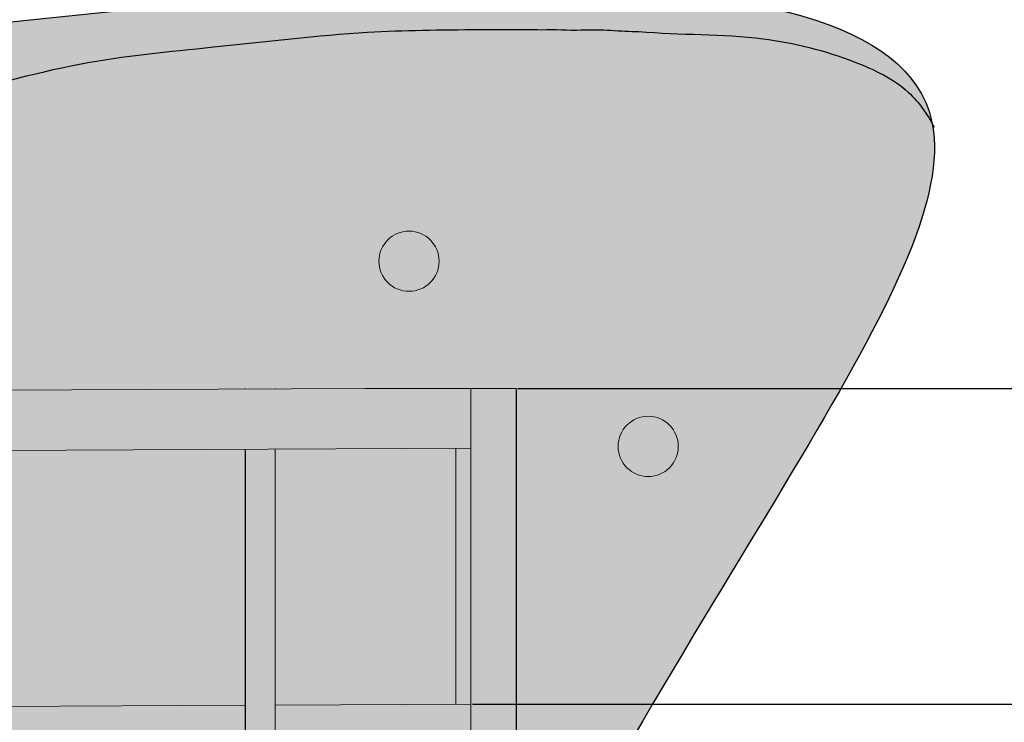
# Model space of a CAD drawing. Units: millimetres. Extents: x 11032 to 26788, y 3406 to 24505.
# Tile 73 of 78: x 21249 to 24519, y 15110 to 17443. Entities that reach past the tile are written whole.
import ezdxf

# ---------------------------------------------------------------- set-up
doc = ezdxf.new("R2010")
doc.units = ezdxf.units.MM
doc.header["$MEASUREMENT"] = 0
for name, color, linetype, lineweight in [('A-ANNO-DIMS', 2, 'Continuous', 18), ('A-GLAZ', 250, 'Continuous', 20), ('A-GLAZ-PATT', 9, 'Continuous', 13), ('A-ROOF', 7, 'Continuous', 30), ('E-LITE', 7, 'Continuous', 18), ('E-LITE-PATT', 7, 'Continuous', 13)]:
    doc.layers.add(name, color=color, linetype=linetype, lineweight=lineweight)
doc.layers.add('A-GLAZ-FRAM-PATT', color=250, linetype='Continuous', lineweight=13, true_color=0x262627)
doc.layers.add('A-ROOF-PATT', color=9, linetype='Continuous', lineweight=13, true_color=0xc7c8ca)
doc.styles.get("Standard").update_dxf_attribs({"font": 'arial.ttf'})
doc.dimstyles.get("Standard").update_dxf_attribs({"dimtxt": 150, "dimasz": 100, "dimexe": 10, "dimexo": 5, "dimgap": 5, "dimtad": 0, "dimtih": 1, "dimtoh": 1, "dimdec": 0, "dimzin": 0, "dimdsep": 46, "dimtxsty": 'Standard', "dimcen": 0.09, "dimadec": 0, "dimazin": 0, "dimtfac": 1, "dimtdec": 0, "dimtofl": 0, "dimtmove": 0, "dimatfit": 3, "dimfxl": 1, "dimtolj": 1, "dimtzin": 0, "dimarcsym": 0})

# ---------------------------------------------------------------- blocks, each defined once
blk = doc.blocks.new('RECESSED-LIGHT-200')
blk.add_circle((100, 100), 100)
blk = doc.blocks.new('*D36')
at = {"layer": 'A-ANNO-DIMS', "color": 0, "lineweight": -2, "transparency": 16777216}
for p, q in [((12301.3, 17115.9), (12301.3, 24416.9)), ((12401.3, 24406.9), (18569.2, 24406.9)), ((25297.4, 24406.9), (19129.5, 24406.9)), ((25397.4, 4466.4), (25397.4, 24416.9))]:
    blk.add_line(p, q, dxfattribs=at)
at = {"layer": 'A-ANNO-DIMS', "color": 0, "transparency": 16777216}
for points in [[(12401.3, 24423.5), (12401.3, 24390.2), (12301.3, 24406.9)], [(25297.4, 24423.5), (25297.4, 24390.2), (25397.4, 24406.9)]]:
    blk.add_solid(points, dxfattribs=at)
at = {"layer": 'Defpoints', "color": 0, "transparency": 16777216}
for p in [(25397.4, 24406.9), (12301.3, 17110.9), (25397.4, 4461.4)]:
    blk.add_point(p, dxfattribs=at)
at = {"layer": 'A-ANNO-DIMS', "color": 0, "transparency": 16777216, "insert": (18849.3, 24406.9), "char_height": 150, "attachment_point": 5}
blk.add_mtext('\\A1;13096', dxfattribs=at)
blk = doc.blocks.new('*D43')
at = {"layer": 'A-ANNO-DIMS', "color": 0, "lineweight": -2, "transparency": 16777216}
for p, q in [((22752.4, 15170.1), (26363.9, 15170.1)), ((26353.9, 15070.1), (26353.9, 14326.7)), ((26353.9, 13420.1), (26353.9, 14163.5)), ((22752.4, 13320.1), (26363.9, 13320.1))]:
    blk.add_line(p, q, dxfattribs=at)
at = {"layer": 'A-ANNO-DIMS', "color": 0, "transparency": 16777216}
for points in [[(26337.2, 15070.1), (26370.6, 15070.1), (26353.9, 15170.1)], [(26337.2, 13420.1), (26370.6, 13420.1), (26353.9, 13320.1)]]:
    blk.add_solid(points, dxfattribs=at)
at = {"layer": 'Defpoints', "color": 0, "transparency": 16777216}
for p in [(22747.4, 15170.1), (26353.9, 15170.1), (22747.4, 13320.1)]:
    blk.add_point(p, dxfattribs=at)
at = {"layer": 'A-ANNO-DIMS', "color": 0, "transparency": 16777216, "insert": (26353.9, 14245.1), "char_height": 150, "attachment_point": 5}
blk.add_mtext('\\A1;1850', dxfattribs=at)
blk = doc.blocks.new('*D44')
at = {"layer": 'A-ANNO-DIMS', "color": 0, "lineweight": -2, "transparency": 16777216}
for p, q in [((22902.4, 16218.4), (26363.9, 16218.4)), ((26353.9, 16118.4), (26353.9, 15775.9)), ((26353.9, 15270.1), (26353.9, 15612.6)), ((22752.4, 15170.1), (26363.9, 15170.1))]:
    blk.add_line(p, q, dxfattribs=at)
at = {"layer": 'A-ANNO-DIMS', "color": 0, "transparency": 16777216}
for points in [[(26337.2, 16118.4), (26370.6, 16118.4), (26353.9, 16218.4)], [(26337.2, 15270.1), (26370.6, 15270.1), (26353.9, 15170.1)]]:
    blk.add_solid(points, dxfattribs=at)
at = {"layer": 'Defpoints', "color": 0, "transparency": 16777216}
for p in [(22897.4, 16218.4), (26353.9, 16218.4), (22747.4, 15170.1)]:
    blk.add_point(p, dxfattribs=at)
at = {"layer": 'A-ANNO-DIMS', "color": 0, "transparency": 16777216, "insert": (26353.9, 15694.3), "char_height": 150, "attachment_point": 5}
blk.add_mtext('\\A1;1048.3', dxfattribs=at)
blk = doc.blocks.new('*D45')
at = {"layer": 'A-ANNO-DIMS', "color": 0, "lineweight": -2, "transparency": 16777216}
for p, q in [((13792.4, 18518.9), (26363.9, 18518.9)), ((26353.9, 18418.9), (26353.9, 17450.3)), ((26353.9, 16318.4), (26353.9, 17287)), ((22902.4, 16218.4), (26363.9, 16218.4))]:
    blk.add_line(p, q, dxfattribs=at)
at = {"layer": 'A-ANNO-DIMS', "color": 0, "transparency": 16777216}
for points in [[(26337.2, 18418.9), (26370.6, 18418.9), (26353.9, 18518.9)], [(26337.2, 16318.4), (26370.6, 16318.4), (26353.9, 16218.4)]]:
    blk.add_solid(points, dxfattribs=at)
at = {"layer": 'Defpoints', "color": 0, "transparency": 16777216}
for p in [(13787.4, 18518.9), (26353.9, 18518.9), (22897.4, 16218.4)]:
    blk.add_point(p, dxfattribs=at)
at = {"layer": 'A-ANNO-DIMS', "color": 0, "transparency": 16777216, "insert": (26353.9, 17368.7), "char_height": 150, "attachment_point": 5}
blk.add_mtext('\\A1;2300.5', dxfattribs=at)
blk = doc.blocks.new('*D51')
at = {"layer": 'A-ANNO-DIMS', "color": 0, "lineweight": -2, "transparency": 16777216}
for p, q in [((19697.4, 16000.7), (19697.4, 3494.9)), ((21997.4, 16011.6), (21997.4, 3494.9)), ((19797.4, 3504.9), (20617.4, 3504.9)), ((21897.4, 3504.9), (21077.4, 3504.9))]:
    blk.add_line(p, q, dxfattribs=at)
at = {"layer": 'A-ANNO-DIMS', "color": 0, "transparency": 16777216}
for points in [[(19797.4, 3521.6), (19797.4, 3488.2), (19697.4, 3504.9)], [(21897.4, 3521.6), (21897.4, 3488.2), (21997.4, 3504.9)]]:
    blk.add_solid(points, dxfattribs=at)
at = {"layer": 'Defpoints', "color": 0, "transparency": 16777216}
for p in [(19697.4, 16005.7), (21997.4, 16016.6), (21997.4, 3504.9)]:
    blk.add_point(p, dxfattribs=at)
at = {"layer": 'A-ANNO-DIMS', "color": 0, "transparency": 16777216, "insert": (20847.4, 3504.9), "char_height": 150, "attachment_point": 5}
blk.add_mtext('\\A1;2300', dxfattribs=at)
blk = doc.blocks.new('*D52')
at = {"layer": 'A-ANNO-DIMS', "color": 0, "lineweight": -2, "transparency": 16777216}
for p, q in [((22897.4, 16213.4), (22897.4, 3494.9)), ((21997.4, 16011.6), (21997.4, 3494.9)), ((22097.4, 3504.9), (22277, 3504.9)), ((22797.4, 3504.9), (22617.9, 3504.9))]:
    blk.add_line(p, q, dxfattribs=at)
at = {"layer": 'A-ANNO-DIMS', "color": 0, "transparency": 16777216}
for points in [[(22097.4, 3521.6), (22097.4, 3488.2), (21997.4, 3504.9)], [(22797.4, 3521.6), (22797.4, 3488.2), (22897.4, 3504.9)]]:
    blk.add_solid(points, dxfattribs=at)
at = {"layer": 'Defpoints', "color": 0, "transparency": 16777216}
for p in [(22897.4, 16218.4), (21997.4, 16016.6), (22897.4, 3504.9)]:
    blk.add_point(p, dxfattribs=at)
at = {"layer": 'A-ANNO-DIMS', "color": 0, "transparency": 16777216, "insert": (22447.4, 3504.9), "char_height": 150, "attachment_point": 5}
blk.add_mtext('\\A1;900', dxfattribs=at)

msp = doc.modelspace()

# ---------------------------------------------------------------- hatches: boundary and pattern name
at = {"layer": 'A-GLAZ-FRAM-PATT'}
h = msp.add_hatch(color=256, dxfattribs=at)
h.paths.add_polyline_path([(22747.404, 16218.44), (22395.025, 16218.44), (18518.2, 16200.148), (18519.143, 16000.151), (22747.404, 16020.1)])
edge = h.paths.add_edge_path()
edge.add_line((22897.404, 16218.44), (22747.404, 16218.44))
edge.add_line((22747.404, 16218.44), (22747.404, 16020.1))
edge.add_line((22747.404, 16020.1), (22747.404, 9631.346))
edge.add_spline(control_points=[(22747.404, 9631.346), (22803.273, 9520.228), (22853.467, 9405.87), (22897.404, 9289.211)], knot_values=[2645.78092422, 2645.78092422, 2645.78092422, 2645.78092422, 3013.05623672, 3013.05623672, 3013.05623672, 3013.05623672], degree=3, periodic=0)
edge.add_line((22897.404, 9289.211), (22897.404, 16218.44))
h.paths.add_polyline_path([(22097.404, 16017.033), (21997.404, 16016.562), (21997.404, 13316.532), (22097.404, 13317.003)])
edge = h.paths.add_edge_path()
edge.add_line((19797.404, 16006.182), (19697.404, 16005.71))
edge.add_line((19697.404, 16005.71), (19697.404, 15155.703))
edge.add_line((19697.404, 15155.703), (19697.404, 12747.012))
edge.add_spline(control_points=[(19697.404, 12747.012), (19708.389, 12750.081), (19719.253, 12753.406), (19732.457, 12757.789), (19734.918, 12758.62), (19737.372, 12759.464)], knot_values=[1372.60477099, 1372.60477099, 1372.60477099, 1372.60477099, 1399.44343377, 1399.44343377, 1405.61279972, 1405.61279972, 1405.61279972, 1405.61279972], degree=3, periodic=0)
edge.add_spline(control_points=[(19737.372, 12759.464), (19750.245, 12763.891), (19762.932, 12768.657), (19778.9, 12775.14), (19782.354, 12776.572), (19785.794, 12778.028)], knot_values=[1405.61279972, 1405.61279972, 1405.61279972, 1405.61279972, 1437.96891336, 1437.96891336, 1446.94640473, 1446.94640473, 1446.94640473, 1446.94640473], degree=3, periodic=0)
edge.add_spline(control_points=[(19785.794, 12778.028), (19789.682, 12779.673), (19793.552, 12781.348), (19797.404, 12783.051)], knot_values=[1446.94640473, 1446.94640473, 1446.94640473, 1446.94640473, 1457.09545574, 1457.09545574, 1457.09545574, 1457.09545574], degree=3, periodic=0)
edge.add_line((19797.404, 12783.051), (19797.404, 15306.174))
edge.add_line((19797.404, 15306.174), (19797.404, 16006.182))
h = msp.add_hatch(color=256, dxfattribs=at)
h.paths.add_polyline_path([(22747.404, 16020.1), (22697.404, 16019.864), (22697.404, 15169.858), (22747.404, 15170.094)])
h.paths.add_polyline_path([(22747.404, 15070.092), (22697.404, 15069.857), (22697.404, 13319.834), (22747.404, 13320.07)])
edge = h.paths.add_edge_path()
edge.add_line((22747.404, 12795.064), (21365.955, 12788.546))
edge.add_spline(control_points=[(21365.955, 12788.546), (21365.556, 12785.216), (21365.14, 12781.894), (21364.707, 12778.582)], knot_values=[4871.89074498, 4871.89074498, 4871.89074498, 4871.89074498, 4881.51384723, 4881.51384723, 4881.51384723, 4881.51384723], degree=3, periodic=0)
edge.add_spline(control_points=[(21364.707, 12778.582), (21363.953, 12772.805), (21363.147, 12767.057), (21359.867, 12745.141), (21357.035, 12729.186), (21353.796, 12713.488)], knot_values=[4881.51384723, 4881.51384723, 4881.51384723, 4881.51384723, 4898.30109774, 4898.30109774, 4945.85686537, 4945.85686537, 4945.85686537, 4945.85686537], degree=3, periodic=0)
edge.add_line((21353.796, 12713.488), (22747.404, 12720.064))
edge.add_line((22747.404, 12720.064), (22747.404, 12795.064))
edge = h.paths.add_edge_path()
edge.add_line((22747.404, 13320.07), (22697.404, 13319.834))
edge.add_line((22697.404, 13319.834), (21312.567, 13313.3))
edge.add_spline(control_points=[(21312.567, 13313.3), (21312.567, 13313.3), (21312.567, 13313.3), (21312.567, 13313.3)], knot_values=[4405.86932069, 4405.86932069, 4405.86932069, 4405.86932069, 4405.86932536, 4405.86932536, 4405.86932536, 4405.86932536], degree=3, periodic=0)
edge.add_spline(control_points=[(21312.567, 13313.3), (21316.329, 13300.292), (21319.935, 13287.252), (21326.522, 13262.273), (21329.53, 13250.337), (21332.397, 13238.393)], knot_values=[4405.86932536, 4405.86932536, 4405.86932536, 4405.86932536, 4439.73791994, 4439.73791994, 4470.65028407, 4470.65028407, 4470.65028407, 4470.65028407], degree=3, periodic=0)
edge.add_line((21332.397, 13238.393), (22747.404, 13245.069))
edge.add_line((22747.404, 13245.069), (22747.404, 13320.07))
h.paths.add_polyline_path([(22747.404, 13245.069), (22697.404, 13244.833), (22697.404, 12794.828), (22747.404, 12795.064)])
h.paths.add_polyline_path([(22747.404, 12720.064), (22697.404, 12719.828), (22697.404, 11219.811), (22747.404, 11220.047)])
edge = h.paths.add_edge_path()
edge.add_line((22747.404, 11120.046), (22697.404, 11119.81))
edge.add_line((22697.404, 11119.81), (22697.404, 9727.135))
edge.add_spline(control_points=[(22697.404, 9727.135), (22714.538, 9695.493), (22731.209, 9663.555), (22747.404, 9631.346)], knot_values=[2539.32128955, 2539.32128955, 2539.32128955, 2539.32128955, 2645.78092422, 2645.78092422, 2645.78092422, 2645.78092422], degree=3, periodic=0)
edge.add_line((22747.404, 9631.346), (22747.404, 11120.046))
h = msp.add_hatch(color=256, dxfattribs=at)
h.paths.add_polyline_path([(19697.404, 15155.703), (18523.154, 15150.163), (18523.626, 15050.164), (19697.404, 15055.702)])
h.paths.add_polyline_path([(21997.404, 15166.555), (19797.404, 15156.175), (19797.404, 15056.174), (20912.335, 15061.434, -0.11801722), (20947.253, 15061.599), (21997.404, 15066.554)])
h.paths.add_polyline_path([(22747.404, 15170.094), (22097.404, 15167.027), (22097.404, 15067.026), (22747.404, 15070.092)])
edge = h.paths.add_edge_path()
edge.add_line((21997.404, 13241.531), (21332.397, 13238.393))
edge.add_spline(control_points=[(21332.397, 13238.393), (21338.038, 13214.902), (21343.139, 13191.382), (21354.5, 13132.481), (21360.029, 13097.149), (21368.306, 13027.119), (21371.052, 12992.421), (21373.63, 12924.101), (21373.462, 12890.481), (21370.61, 12834.187), (21368.665, 12811.15), (21365.955, 12788.546)], knot_values=[4470.65028407, 4470.65028407, 4470.65028407, 4470.65028407, 4531.4505555, 4531.4505555, 4623.16319106, 4623.16319106, 4714.87582662, 4714.87582662, 4806.58846218, 4806.58846218, 4871.89074498, 4871.89074498, 4871.89074498, 4871.89074498], degree=3, periodic=0)
edge.add_line((21365.955, 12788.546), (21997.404, 12791.526))
edge.add_line((21997.404, 12791.526), (21997.404, 13241.531))
h.paths.add_polyline_path([(22097.404, 13242.003), (21997.404, 13241.531), (21997.404, 12791.526), (22097.404, 12791.998)])
h.paths.add_polyline_path([(22697.404, 13244.833), (22097.404, 13242.003), (22097.404, 12791.998), (22697.404, 12794.828)])
at = {"layer": 'A-GLAZ-PATT'}
h = msp.add_hatch(color=256, dxfattribs=at)
h.set_gradient(color1=(254, 221, 154), color2=(248, 246, 176), name='CURVED')
edge = h.paths.add_edge_path()
edge.add_spline(control_points=[(18522.918, 15200.175), (18561.599, 15201.209), (18600.224, 15202.243), (18716.594, 15205.749), (18794.099, 15208.613), (18948.086, 15217.451), (19024.568, 15223.425), (19176.135, 15240.511), (19251.219, 15251.623), (19333.848, 15267.966), (19342.25, 15269.676), (19356.967, 15272.758), (19363.289, 15274.111), (19375.94, 15276.871), (19382.267, 15278.279), (19401.252, 15282.576), (19413.915, 15285.541), (19451.935, 15294.685), (19477.322, 15301.111), (19548.254, 15319.552), (19593.948, 15331.984), (19659.079, 15349.253), (19678.203, 15354.269), (19697.404, 15359.188)], knot_values=[1.09285599, 1.09285599, 1.09285599, 1.09285599, 116.34451384, 116.34451384, 349.03354152, 349.03354152, 581.72256921, 581.72256921, 814.41159689, 814.41159689, 840.78637359, 840.78637359, 860.67891922, 860.67891922, 880.57146485, 880.57146485, 920.35655611, 920.35655611, 999.92673863, 999.92673863, 1142.09604805, 1142.09604805, 1200.90860694, 1200.90860694, 1200.90860694, 1200.90860694], degree=3, periodic=0)
edge.add_line((19697.404, 15359.188), (19697.404, 16005.71))
edge.add_line((19697.404, 16005.71), (18519.143, 16000.151))
edge.add_line((18519.143, 16000.151), (18522.918, 15200.175))
edge = h.paths.add_edge_path()
edge.add_line((19697.404, 15055.702), (18523.626, 15050.164))
edge.add_line((18523.626, 15050.164), (18531.851, 13306.733))
edge.add_spline(control_points=[(18531.851, 13306.733), (18553.325, 13284.933), (18574.901, 13263.301), (18632.771, 13206.214), (18669.261, 13171.188), (18735.852, 13109.762), (18765.813, 13083.011), (18826.398, 13031.156), (18857.021, 13006.052), (18919.15, 12957.862), (18950.655, 12934.774), (19007.615, 12895.967), (19032.834, 12879.759), (19084.165, 12849.05), (19110.278, 12834.547), (19163.6, 12807.555), (19190.811, 12795.065), (19240.068, 12775.123), (19261.85, 12767.175), (19306.233, 12752.949), (19328.834, 12746.672), (19374.859, 12736.071), (19398.283, 12731.748), (19445.866, 12725.365), (19470.026, 12723.306), (19514.597, 12721.889), (19534.921, 12722.121), (19575.756, 12724.466), (19596.267, 12726.579), (19622.683, 12730.57), (19628.6, 12731.546), (19638.601, 12733.337), (19642.688, 12734.108), (19650.826, 12735.723), (19654.881, 12736.567), (19667.001, 12739.207), (19675.023, 12741.111), (19687.813, 12744.388), (19692.62, 12745.676), (19697.404, 12747.012)], knot_values=[259.28299856, 259.28299856, 259.28299856, 259.28299856, 332.45020059, 332.45020059, 454.53383699, 454.53383699, 552.84889009, 552.84889009, 651.16394319, 651.16394319, 749.47899629, 749.47899629, 825.6298474, 825.6298474, 901.7806985, 901.7806985, 977.9315496, 977.9315496, 1036.43952646, 1036.43952646, 1094.94750331, 1094.94750331, 1153.45548017, 1153.45548017, 1211.96345702, 1211.96345702, 1260.21270617, 1260.21270617, 1308.46195531, 1308.46195531, 1322.39247458, 1322.39247458, 1332.02384448, 1332.02384448, 1341.65521438, 1341.65521438, 1360.91795418, 1360.91795418, 1372.60477099, 1372.60477099, 1372.60477099, 1372.60477099], degree=3, periodic=0)
edge.add_line((19697.404, 12747.012), (19697.404, 15055.702))
h.paths.add_polyline_path([(18790.086, 14298.34, -1), (18890.086, 14298.34, -1)], flags=16)
h.paths.add_polyline_path([(19437.524, 14550.125, -1), (19537.524, 14550.125, -1)], flags=16)
h.paths.add_polyline_path([(22697.404, 16019.864), (22097.404, 16017.033), (22097.404, 15167.027), (22697.404, 15169.858)])
h.paths.add_polyline_path([(22697.404, 15069.857), (22097.404, 15067.026), (22097.404, 13317.003), (22697.404, 13319.834)])
h.paths.add_polyline_path([(20866.429, 15795.606, -1), (21016.429, 15795.606, -1)], flags=16)
h.paths.add_polyline_path([(19822.441, 15337.78), (19797.404, 15332.147), (19797.404, 15156.175), (20721.869, 15160.537), (20700.803, 15175.665), (20679.512, 15190.548), (20657.993, 15205.143), (20636.247, 15219.41), (20614.273, 15233.307), (20592.07, 15246.794), (20569.639, 15259.829), (20546.978, 15272.372), (20524.088, 15284.38), (20500.968, 15295.814), (20477.616, 15306.631), (20454.034, 15316.792), (20430.219, 15326.254), (20406.173, 15334.976), (20381.894, 15342.919), (20357.382, 15350.039), (20332.636, 15356.297), (20307.662, 15361.667), (20282.483, 15366.173), (20257.125, 15369.849), (20231.617, 15372.729), (20205.984, 15374.847), (20180.253, 15376.236), (20154.451, 15376.931), (20128.605, 15376.964), (20102.742, 15376.37), (20076.889, 15375.183), (20051.072, 15373.436), (20025.318, 15371.163), (19999.653, 15368.398), (19974.087, 15365.173), (19948.614, 15361.516), (19923.228, 15357.456), (19897.924, 15353.024), (19872.695, 15348.248), (19847.536, 15343.157)])
h.paths.add_polyline_path([(19797.404, 15383.428), (19822.666, 15388.998), (19848.044, 15394.311), (19873.542, 15399.338), (19899.168, 15404.048), (19924.927, 15408.41), (19950.824, 15412.396), (19976.865, 15415.972), (20003.054, 15419.109), (20029.394, 15421.774), (20055.871, 15423.934), (20082.461, 15425.553), (20109.142, 15426.594), (20135.888, 15427.02), (20162.676, 15426.794), (20189.481, 15425.88), (20216.28, 15424.237), (20243.046, 15421.828), (20269.754, 15418.614), (20296.377, 15414.554), (20322.887, 15409.61), (20349.254, 15403.74), (20375.368, 15396.947), (20401.163, 15389.283), (20426.64, 15380.795), (20451.799, 15371.531), (20476.643, 15361.538), (20501.172, 15350.863), (20525.391, 15339.55), (20549.302, 15327.645), (20572.91, 15315.192), (20596.218, 15302.234), (20619.229, 15288.816), (20641.948, 15274.978), (20664.378, 15260.764), (20686.523, 15246.215), (20708.386, 15231.373), (20729.97, 15216.279), (20751.277, 15200.974), (20806.33, 15160.935), (21997.404, 15166.555), (21997.404, 16016.562), (19797.404, 16006.182)])
at = {"layer": 'A-ROOF-PATT'}
h = msp.add_hatch(color=256, dxfattribs=at)
edge = h.paths.add_edge_path()
edge.add_spline(control_points=[(18514.126, 17063.566), (18809.773, 17038.521), (19288.07, 16988.339), (19761.843, 17020.464), (19965.955, 17031.58)], knot_values=[0, 0, 0, 0, 871.48115533, 1383.18424693, 1383.18424693, 1383.18424693, 1383.18424693], degree=3, periodic=0)
edge.add_spline(control_points=[(19965.955, 17031.58), (20122.484, 17046.068), (20408.011, 17091.181), (20910.567, 17150.246), (21440.234, 17310.172), (21915.866, 17351.508), (22364.272, 17406.622), (22705.353, 17409.356), (22912.577, 17410.967), (22981.194, 17409.426)], knot_values=[0, 0, 0, 0, 414.81784697, 1085.22788952, 1556.54039253, 2003.31216232, 2520.51919616, 2899.47011217, 3092.27759325, 3092.27759325, 3092.27759325, 3092.27759325], degree=3, periodic=0)
edge.add_spline(control_points=[(22981.194, 17409.426), (23026.355, 17412.719), (23070.675, 17406.134), (23179.968, 17412.17), (23244.326, 17403.734), (23304.873, 17403.391)], knot_values=[11756.28081343, 11756.28081343, 11756.28081343, 11756.28081343, 11879.15309498, 11879.15309498, 12065.87545546, 12065.87545546, 12065.87545546, 12065.87545546], degree=3, periodic=0)
edge.add_spline(control_points=[(23304.873, 17403.391), (23443.416, 17391.278), (23687.5, 17400.339), (23988.629, 17323.661), (24193.084, 17226.949), (24257.37, 17136.735), (24279.347, 17098.191)], knot_values=[0, 0, 0, 0, 412.75172359, 727.19040018, 931.86025321, 1064.01641738, 1064.01641738, 1064.01641738, 1064.01641738], degree=3, periodic=0)
edge.add_spline(control_points=[(24279.347, 17098.191), (24276.632, 17112.026), (24103.56, 17784.539), (21679.83, 17482.933), (20092.886, 17311.864), (19886.51, 17298.161)], knot_values=[9435.32329041, 9435.32329041, 9435.32329041, 9435.32329041, 9511.54858978, 13244.41643911, 13837.11981978, 13837.11981978, 13837.11981978, 13837.11981978], degree=3, periodic=0)
edge.add_spline(control_points=[(19886.51, 17298.161), (19770.33, 17290.447), (19654.15, 17282.732), (19537.97, 17275.018), (19460.41, 17269.868), (19382.851, 17264.718), (19305.291, 17259.568)], knot_values=[8878.9087223, 8878.9087223, 8878.9087223, 8878.9087223, 9212.57342317, 9212.57342317, 9212.57342317, 9435.32303857, 9435.32303857, 9435.32303857, 9435.32303857], degree=3, periodic=0)
edge.add_spline(control_points=[(19305.291, 17259.568), (19183.371, 17255.041), (18919.19, 17257.277), (18655.158, 17260.282), (18513.182, 17263.662)], knot_values=[568.98430855, 568.98430855, 568.98430855, 568.98430855, 934.97323186, 1361.07600794, 1361.07600794, 1361.07600794, 1361.07600794], degree=3, periodic=0)
edge.add_line((18513.182, 17263.662), (18514.126, 17063.566))
h = msp.add_hatch(color=256, dxfattribs=at)
h.set_gradient(color1=(254, 234, 185), color2=(254, 204, 102), name='HEMISPHERICAL')
edge = h.paths.add_edge_path()
edge.add_line((22395.025, 16218.44), (22897.404, 16218.44))
edge.add_line((22897.404, 16218.44), (22897.404, 14361.22))
edge.add_spline(control_points=[(22897.404, 14361.22), (23633.498, 15762.375), (24369.592, 16638.387), (24279.347, 17098.191)], knot_values=[13837.11981978, 13837.11981978, 13837.11981978, 13837.11981978, 16370.50452639, 16370.50452639, 16370.50452639, 16370.50452639], degree=3, periodic=0)
edge.add_spline(control_points=[(24279.347, 17098.191), (24257.37, 17136.735), (24193.084, 17226.949), (23988.629, 17323.661), (23687.5, 17400.339), (23443.416, 17391.278), (23304.873, 17403.391)], knot_values=[0, 0, 0, 0, 132.15616417, 336.8260172, 651.2646938, 1064.01641738, 1064.01641738, 1064.01641738, 1064.01641738], degree=3, periodic=0)
edge.add_spline(control_points=[(23304.873, 17403.391), (23244.326, 17403.734), (23179.968, 17412.17), (23070.675, 17406.134), (23026.355, 17412.719), (22981.194, 17409.426)], knot_values=[11756.28081343, 11756.28081343, 11756.28081343, 11756.28081343, 11943.0031739, 11943.0031739, 12065.87545546, 12065.87545546, 12065.87545546, 12065.87545546], degree=3, periodic=0)
edge.add_spline(control_points=[(22981.194, 17409.426), (22912.577, 17410.967), (22705.353, 17409.356), (22364.272, 17406.622), (21915.866, 17351.508), (21440.234, 17310.172), (20910.567, 17150.246), (20408.011, 17091.181), (20122.484, 17046.068), (19965.955, 17031.58)], knot_values=[0, 0, 0, 0, 192.80748108, 571.75839709, 1088.96543094, 1535.73720072, 2007.04970373, 2677.45974628, 3092.27759325, 3092.27759325, 3092.27759325, 3092.27759325], degree=3, periodic=0)
edge.add_spline(control_points=[(19965.955, 17031.58), (19761.843, 17020.464), (19288.07, 16988.339), (18809.773, 17038.521), (18514.126, 17063.566)], knot_values=[0, 0, 0, 0, 511.7030916, 1383.18424693, 1383.18424693, 1383.18424693, 1383.18424693], degree=3, periodic=0)
edge.add_line((18514.126, 17063.566), (18518.2, 16200.148))
edge.add_line((18518.2, 16200.148), (22395.025, 16218.44))
h.paths.add_polyline_path([(20159.481, 16629.671, -1), (20359.481, 16629.671, -1)], flags=16)
h.paths.add_polyline_path([(22641.869, 16640.848, -1), (22441.869, 16640.848, -1)], flags=16)
h.paths.add_polyline_path([(23436.23, 16026.079, -1), (23236.23, 16026.079, -1)], flags=16)
at = {"layer": 'E-LITE-PATT'}
h = msp.add_hatch(color=256, dxfattribs=at)
edge = h.paths.add_edge_path()
edge.add_spline(control_points=[(18523.154, 15150.163), (18807.347, 15157.761), (19206.112, 15168.423), (19587.098, 15279.026), (19697.404, 15307.557)], knot_values=[0, 0, 0, 0, 846.75149574, 1188.1141131, 1188.1141131, 1188.1141131, 1188.1141131], degree=3, periodic=0)
edge.add_line((19697.404, 15307.557), (19697.404, 15359.188))
edge.add_spline(control_points=[(19697.404, 15359.188), (19678.203, 15354.269), (19659.079, 15349.253), (19593.948, 15331.984), (19548.254, 15319.552), (19477.322, 15301.111), (19451.935, 15294.685), (19413.915, 15285.541), (19401.252, 15282.576), (19382.267, 15278.279), (19375.94, 15276.871), (19363.289, 15274.111), (19356.967, 15272.758), (19342.25, 15269.676), (19333.848, 15267.966), (19251.219, 15251.623), (19176.135, 15240.511), (19024.568, 15223.425), (18948.086, 15217.451), (18794.099, 15208.613), (18716.594, 15205.749), (18600.224, 15202.243), (18561.599, 15201.209), (18522.918, 15200.175)], knot_values=[1.09285599, 1.09285599, 1.09285599, 1.09285599, 59.90541488, 59.90541488, 202.0747243, 202.0747243, 281.64490682, 281.64490682, 321.42999808, 321.42999808, 341.32254371, 341.32254371, 361.21508934, 361.21508934, 387.58986604, 387.58986604, 620.27889372, 620.27889372, 852.96792141, 852.96792141, 1085.65694909, 1085.65694909, 1200.90860694, 1200.90860694, 1200.90860694, 1200.90860694], degree=3, periodic=0)
edge.add_line((18522.918, 15200.175), (18523.154, 15150.163))
edge = h.paths.add_edge_path()
edge.add_spline(control_points=[(19797.404, 15332.147), (19868.636, 15348.527), (20045.965, 15382.128), (20379.232, 15379.049), (20603.72, 15246.463), (20721.869, 15160.537)], knot_values=[1290.96802179, 1290.96802179, 1290.96802179, 1290.96802179, 1509.98304384, 1831.38750258, 2265.00925431, 2265.00925431, 2265.00925431, 2265.00925431], degree=3, periodic=0)
edge.add_line((20721.869, 15160.537), (20806.33, 15160.935))
edge.add_spline(control_points=[(20806.33, 15160.935), (20787.979, 15174.281), (20769.629, 15187.627), (20751.278, 15200.973), (20751.278, 15200.973), (20751.277, 15200.974), (20751.277, 15200.974)], knot_values=[2265.00925431, 2265.00925431, 2265.00925431, 2265.00925431, 2330.89307837, 2330.89307837, 2330.89307837, 2330.89358007, 2330.89358007, 2330.89358007, 2330.89358007], degree=3, periodic=0)
edge.add_spline(control_points=[(20751.277, 15200.974), (20751.247, 15200.996), (20751.217, 15201.018), (20722.252, 15222.081), (20692.553, 15242.645), (20631.556, 15281.877), (20600.258, 15300.544), (20535.977, 15335.007), (20502.992, 15350.803), (20448.844, 15372.942), (20428.246, 15380.535), (20396.869, 15390.701), (20386.329, 15393.886), (20370.401, 15398.335), (20365.072, 15399.763), (20354.373, 15402.506), (20349.001, 15403.822), (20337.544, 15406.494), (20331.459, 15407.834), (20315.169, 15411.216), (20304.944, 15413.125), (20281.909, 15416.972), (20269.086, 15418.802), (20222.263, 15424.425), (20188.116, 15426.504), (20124.362, 15427.321), (20094.738, 15426.456), (20050.592, 15423.632), (20035.925, 15422.435), (20006.724, 15419.587), (19992.193, 15417.937), (19959.175, 15413.705), (19940.732, 15410.994), (19880.215, 15401.109), (19838.589, 15392.722), (19797.404, 15383.428)], knot_values=[1302.24166378, 1302.24166378, 1302.24166378, 1302.24166378, 1302.35087893, 1302.35087893, 1406.225269, 1406.225269, 1510.09965908, 1510.09965908, 1613.97404916, 1613.97404916, 1676.17986117, 1676.17986117, 1707.28276717, 1707.28276717, 1722.83422018, 1722.83422018, 1738.38567318, 1738.38567318, 1755.91676333, 1755.91676333, 1785.22951081, 1785.22951081, 1821.79065604, 1821.79065604, 1918.47644845, 1918.47644845, 2002.64679624, 2002.64679624, 2044.73197014, 2044.73197014, 2086.81714404, 2086.81714404, 2140.81625119, 2140.81625119, 2265.00925431, 2265.00925431, 2265.00925431, 2265.00925431], degree=3, periodic=0)
edge.add_line((19797.404, 15383.428), (19797.404, 15332.147))
h.paths.add_polyline_path([(21016.429, 15795.606, 1), (20866.429, 15795.606, 1)])
h.paths.add_polyline_path([(23236.23, 16026.079, 1), (23436.23, 16026.079, 1)])
h.paths.add_polyline_path([(22441.869, 16640.848, 1), (22641.869, 16640.848, 1)])
h.paths.add_polyline_path([(20159.481, 16629.671, 1), (20359.481, 16629.671, 1)])

# ---------------------------------------------------------------- linework, layer by layer
at = {"layer": 'A-GLAZ'}
for p, q in [((22395.025, 16218.44), (18518.2, 16200.148)), ((21997.404, 16218.44), (21997.404, 16216.564)), ((22097.404, 16218.44), (22097.404, 16217.036)), ((22897.404, 16218.44), (22395.025, 16218.44)), ((22747.404, 16218.44), (22747.404, 9631.346)), ((22897.404, 16218.44), (22897.404, 9289.211)), ((22747.404, 16020.1), (18519.143, 16000.151)), ((21997.404, 16016.562), (21997.404, 13316.532)), ((22097.404, 16017.033), (22097.404, 13317.003)), ((22697.404, 16019.864), (22697.404, 15169.858)), ((22697.404, 15319.857), (22697.404, 15169.858)), ((21997.404, 15166.555), (19797.404, 15156.175)), ((22747.404, 15170.094), (22097.404, 15167.027))]:
    msp.add_line(p, q, dxfattribs=at)
at = {"layer": 'A-ROOF'}
for points, knots in [([(19305.291, 17259.568), (19382.851, 17264.718), (19460.41, 17269.868), (19537.97, 17275.018), (19654.15, 17282.732), (19770.33, 17290.447), (19886.51, 17298.161), (19886.51, 17298.161), (19886.51, 17298.161), (19886.51, 17298.161), (20092.886, 17311.864), (21679.83, 17482.933), (25498.5, 17958.124), (23655.645, 15804.534), (22897.404, 14361.22)], [8878.9087223, 8878.9087223, 8878.9087223, 8878.9087223, 9101.65833771, 9101.65833771, 9101.65833771, 9435.32303857, 9435.32303857, 9435.32303857, 9435.32329041, 9435.32329041, 9435.32329041, 10028.02667108, 13760.8945204, 16370.50452639, 16370.50452639, 16370.50452639, 16370.50452639]), ([(19965.955, 17031.58), (20122.484, 17046.068), (20408.011, 17091.181), (20910.567, 17150.246), (21440.234, 17310.172), (21915.866, 17351.508), (22364.272, 17406.622), (22705.353, 17409.356), (22912.577, 17410.967), (22981.194, 17409.426)], [0, 0, 0, 0, 414.81784697, 1085.22788952, 1556.54039253, 2003.31216232, 2520.51919616, 2899.47011217, 3092.27759325, 3092.27759325, 3092.27759325, 3092.27759325]), ([(22981.194, 17409.426), (23026.355, 17412.719), (23070.675, 17406.134), (23179.968, 17412.17), (23244.326, 17403.734), (23304.873, 17403.391)], [11756.28081343, 11756.28081343, 11756.28081343, 11756.28081343, 11879.15309498, 11879.15309498, 12065.87545546, 12065.87545546, 12065.87545546, 12065.87545546]), ([(23304.873, 17403.391), (23443.416, 17391.278), (23687.5, 17400.339), (23988.629, 17323.661), (24197.566, 17224.829), (24262.745, 17129.016), (24286.359, 17085.594)], [0, 0, 0, 0, 412.75172359, 727.19040018, 931.86025321, 1078.29214041, 1078.29214041, 1078.29214041, 1078.29214041])]:
    msp.add_open_spline(points, degree=3, knots=knots, dxfattribs=at)

# ---------------------------------------------------------------- block references
at = {"layer": 'E-LITE'}
for p in [(22441.869, 16540.848), (23236.229, 15926.079)]:
    msp.add_blockref('RECESSED-LIGHT-200', p, dxfattribs=at)

# ---------------------------------------------------------------- dimensions: what is measured, and where the dimension line sits
at = {"layer": 'A-ANNO-DIMS'}
for base, p1, p2, picture, middle in [((25397.404, 24406.858), (12301.265, 17110.885), (25397.404, 4461.399), '*D36', (18849.334, 24406.858)), ((22897.404, 3504.899), (21997.404, 16016.562), (22897.404, 16218.44), '*D52', (22447.404, 3504.899)), ((21997.404, 3504.899), (19697.404, 16005.71), (21997.404, 16016.562), '*D51', (20847.404, 3504.899))]:
    dim = msp.add_linear_dim(base=base, p1=p1, p2=p2, dimstyle='Standard', override={"dimdec": 0, "dimlfac": 1, "dimrnd": 0, "dimzin": 0, "dimdsep": 46, "dimlunit": 2}, dxfattribs=at)
    dim.commit()
    dim.dimension.update_dxf_attribs({"geometry": picture, "text_midpoint": middle})
for base, p1, p2, override, picture, middle in [((26353.904, 18518.925), (22897.404, 16218.44), (13787.367, 18518.925), {"dimdec": 1, "dimlfac": 1, "dimrnd": 0, "dimzin": 0, "dimdsep": 46, "dimlunit": 2}, '*D45', (26353.904, 17368.682)), ((26353.904, 16218.44), (22747.404, 15170.094), (22897.404, 16218.44), {"dimdec": 1, "dimlfac": 1, "dimrnd": 0, "dimzin": 0, "dimdsep": 46, "dimlunit": 2}, '*D44', (26353.904, 15694.267)), ((26353.904, 15170.094), (22747.404, 13320.07), (22747.404, 15170.094), {"dimdec": 0, "dimlfac": 1, "dimrnd": 0, "dimzin": 0, "dimdsep": 46, "dimlunit": 2}, '*D43', (26353.904, 14245.082))]:
    dim = msp.add_linear_dim(base=base, p1=p1, p2=p2, angle=90, dimstyle='Standard', override=override, dxfattribs=at)
    dim.commit()
    dim.dimension.update_dxf_attribs({"geometry": picture, "text_midpoint": middle})

doc.saveas('drawing.dxf')
